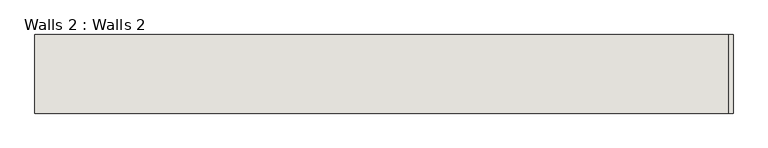
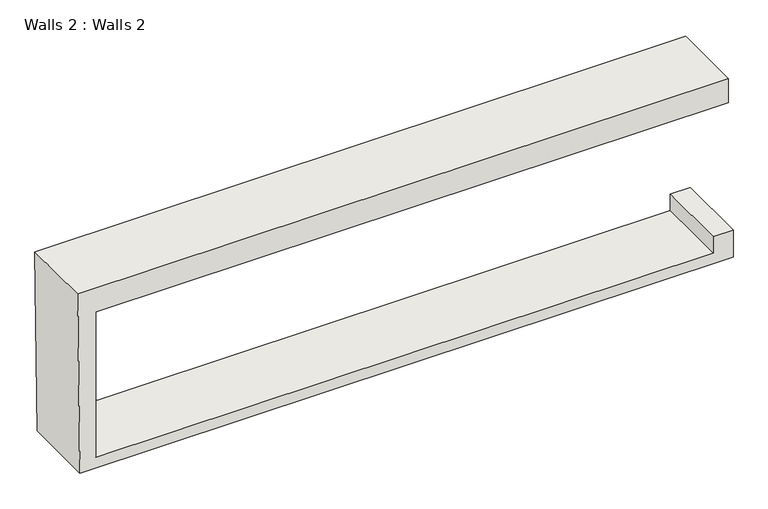
"""IFC4 building model written with IfcOpenShell, lengths in millimetres: wall geometry, Walls 2 : Walls 2."""

from ifc_helpers import new_model, si_unit, frame, origin, place, context, project, spatial, polyline, outline, extrude, source, transform, mapped, element, save


def walls_2_walls_2_9d43e08d(model_context):
    return source(origin(), model_context, "Body", "SweptSolid", [
        extrude(outline(polyline([(14096.0, 10309.98018), (14096.0, -17991.4489699), (5813.8746102, -17886.4428527), (5813.8746102, 10509.98018), (7068.7210408, 10509.98018), (7068.7210408, 9637.5984928), (6308.7210408, 9637.5984928), (6308.7210408, -17190.01982), (12992.5933327, -17190.01982), (12992.5933327, 10309.98018), (14096.0, 10309.98018)])), frame((0.0, -11041.3951407, 0.0), z_axis=(0.0, 1.0, 0.0), x_axis=(0.0, 0.0, 1.0)), (0.0, 0.0, 1.0), 3208.498578),
    ])


if __name__ == "__main__":
    model = new_model("IFC4")
    model_context = context("Model", 3, world=origin())
    ifc_project = project(units=[si_unit("LENGTHUNIT", "METRE", prefix="MILLI")], contexts=[model_context])
    site = spatial("IfcSite", under=ifc_project)
    building = spatial("IfcBuilding", under=site)
    placement = place(None, origin())
    walls_2_walls_2_shape = walls_2_walls_2_9d43e08d(model_context)
    element("IfcWall", 1, ObjectType="Walls 2 : Walls 2", at=placement, inside=building, context=model_context, shape_type="MappedRepresentation", body=[
        mapped(walls_2_walls_2_shape, transform((0.0, 0.0, 0.0), x_axis=(1.0, 0.0, 0.0), y_axis=(0.0, 1.0, 0.0), z_axis=(0.0, 0.0, 1.0))),
    ])
    save(model, "model.ifc")

# Revit data of these elements
# Element 1 (IfcWall, "Walls 2 : Walls 2")
#   Materials on its faces: "Default Wall"
# Materials
#   "Default Wall": colour RGB 80 80 80, transparency 0
